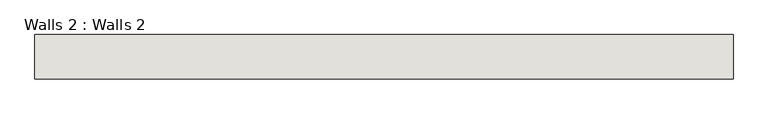
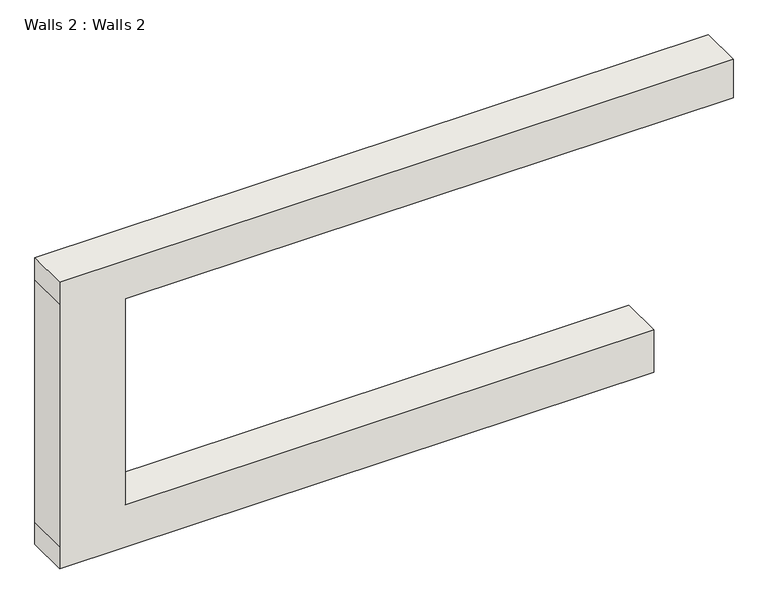
"""IFC4 building model written with IfcOpenShell, lengths in millimetres: wall geometry, Walls 2 : Walls 2."""

from ifc_helpers import new_model, si_unit, frame, origin, place, context, project, spatial, polyline, outline, extrude, source, transform, mapped, element, save


def walls_2_walls_2_beab6565(model_context):
    return source(origin(), model_context, "Body", "SweptSolid", [
        extrude(outline(polyline([(7620.0, -4240.8390038), (7620.0, -13056.0707328), (7315.2, -13056.0707328), (3962.4, -13056.0707328), (3657.6, -13056.0707328), (3657.6, -5281.411895), (4246.5363771, -5281.411895), (4246.5363771, -12199.3933182), (7091.4640657, -12199.3933182), (7091.4640657, -4240.8390038), (7620.0, -4240.8390038)])), frame((0.0, -1335.8574077, 0.0), z_axis=(0.0, 1.0, 0.0), x_axis=(0.0, 0.0, 1.0)), (0.0, 0.0, 1.0), 558.8),
    ])


if __name__ == "__main__":
    model = new_model("IFC4")
    model_context = context("Model", 3, world=origin())
    ifc_project = project(units=[si_unit("LENGTHUNIT", "METRE", prefix="MILLI")], contexts=[model_context])
    site = spatial("IfcSite", under=ifc_project)
    building = spatial("IfcBuilding", under=site)
    placement = place(None, origin())
    walls_2_walls_2_shape = walls_2_walls_2_beab6565(model_context)
    element("IfcWall", 1, ObjectType="Walls 2 : Walls 2", at=placement, inside=building, context=model_context, shape_type="MappedRepresentation", body=[
        mapped(walls_2_walls_2_shape, transform((0.0, 0.0, 0.0), x_axis=(1.0, 0.0, 0.0), y_axis=(0.0, 1.0, 0.0), z_axis=(0.0, 0.0, 1.0))),
    ])
    save(model, "model.ifc")

# Revit data of these elements
# Element 1 (IfcWall, "Walls 2 : Walls 2")
#   Materials on its faces: "Default Wall"
# Materials
#   "Default Wall": colour RGB 128 128 128, transparency 0
